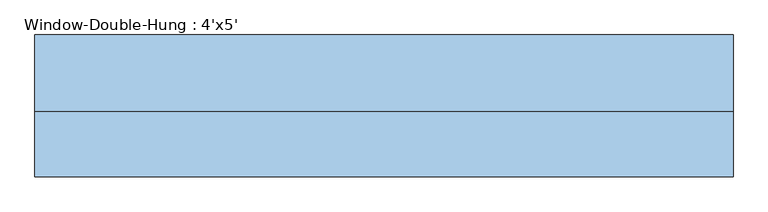
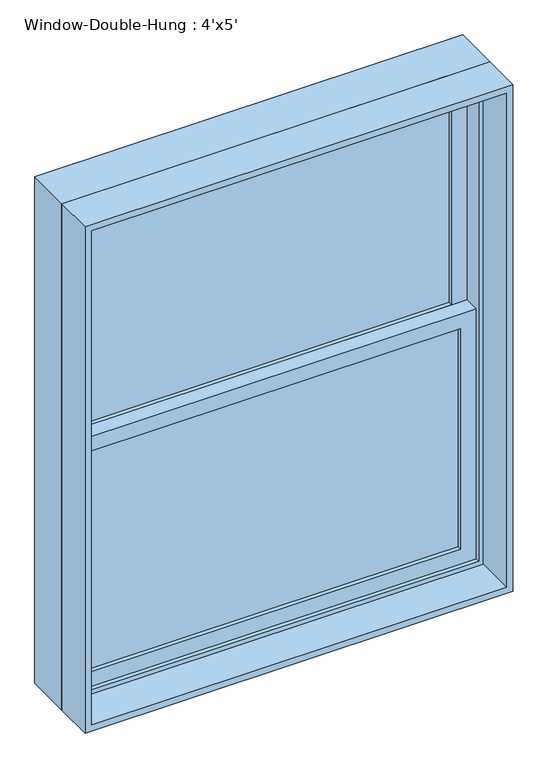
"""IFC4 building model written with IfcOpenShell, lengths in millimetres: window geometry, Window-Double-Hung : 4'x5'."""

from ifc_helpers import new_model, si_unit, frame, origin, place, context, project, spatial, polyline, outline, extrude, source, transform, mapped, element, save


def window_double_hung_4_x5_5ded1df2(model_context):
    return source(origin(), model_context, "Body", "SweptSolid", [
        extrude(outline(polyline([(533.4, 44.45), (533.4, 38.1), (-533.4, 38.1), (-533.4, 44.45), (533.4, 44.45)])), frame((0.0, 0.0, 990.6), z_axis=(0.0, 0.0, 1.0), x_axis=(1.0, 0.0, 0.0)), (0.0, 0.0, 1.0), 663.575),
        extrude(outline(polyline([(-533.4, 31.75), (533.4, 31.75), (533.4, 25.4), (-533.4, 25.4), (-533.4, 31.75)])), frame((0.0, 0.0, 990.6), z_axis=(0.0, 0.0, 1.0), x_axis=(1.0, 0.0, 0.0)), (0.0, 0.0, 1.0), 663.575),
        extrude(outline(polyline([(533.4, 88.9), (533.4, 82.55), (-533.4, 82.55), (-533.4, 88.9), (533.4, 88.9)])), frame((0.0, 0.0, 1698.625), z_axis=(0.0, 0.0, 1.0), x_axis=(1.0, 0.0, 0.0)), (0.0, 0.0, 1.0), 663.575),
        extrude(outline(polyline([(-533.4, 76.2), (533.4, 76.2), (533.4, 69.85), (-533.4, 69.85), (-533.4, 76.2)])), frame((0.0, 0.0, 1698.625), z_axis=(0.0, 0.0, 1.0), x_axis=(1.0, 0.0, 0.0)), (0.0, 0.0, 1.0), 663.575),
        extrude(outline(polyline([(1698.625, -577.85), (946.15, -577.85), (946.15, 577.85), (1698.625, 577.85), (1698.625, -577.85)]), holes=[polyline([(1654.175, 533.4), (990.6, 533.4), (990.6, -533.4), (1654.175, -533.4), (1654.175, 533.4)])]), frame((0.0, 12.7, 0.0), z_axis=(0.0, 1.0, 0.0), x_axis=(0.0, 0.0, 1.0)), (0.0, 0.0, 1.0), 44.45),
        extrude(outline(polyline([(2406.65, -577.85), (1654.175, -577.85), (1654.175, 577.85), (2406.65, 577.85), (2406.65, -577.85)]), holes=[polyline([(2362.2, 533.4), (1698.625, 533.4), (1698.625, -533.4), (2362.2, -533.4), (2362.2, 533.4)])]), frame((0.0, 57.15, 0.0), z_axis=(0.0, 1.0, 0.0), x_axis=(0.0, 0.0, 1.0)), (0.0, 0.0, 1.0), 44.45),
        extrude(outline(polyline([(2438.4, -609.6), (914.4, -609.6), (914.4, 609.6), (2438.4, 609.6), (2438.4, -609.6)]), holes=[polyline([(2406.65, 577.85), (946.15, 577.85), (946.15, -577.85), (2406.65, -577.85), (2406.65, 577.85)])]), frame((0.0, 0.0, 0.0), z_axis=(0.0, 1.0, 0.0), x_axis=(0.0, 0.0, 1.0)), (0.0, 0.0, 1.0), 133.35),
        extrude(outline(polyline([(2438.4, 609.6), (2438.4, -609.6), (914.4, -609.6), (914.4, 609.6), (2438.4, 609.6)]), holes=[polyline([(2419.35, 590.55), (933.45, 590.55), (933.45, -590.55), (2419.35, -590.55), (2419.35, 590.55)])]), frame((0.0, -114.3, 0.0), z_axis=(0.0, 1.0, 0.0), x_axis=(0.0, 0.0, 1.0)), (0.0, 0.0, 1.0), 114.3),
    ])


if __name__ == "__main__":
    model = new_model("IFC4")
    model_context = context("Model", 3, world=origin())
    ifc_project = project(units=[si_unit("LENGTHUNIT", "METRE", prefix="MILLI")], contexts=[model_context])
    site = spatial("IfcSite", under=ifc_project)
    building = spatial("IfcBuilding", under=site)
    placement = place(None, origin())
    window_double_hung_4_x5_shape = window_double_hung_4_x5_5ded1df2(model_context)
    element("IfcWindow", 1, ObjectType="Window-Double-Hung : 4'x5'", at=placement, inside=building, context=model_context, shape_type="MappedRepresentation", body=[
        mapped(window_double_hung_4_x5_shape, transform((0.0, 0.0, 0.0), x_axis=(1.0, 0.0, 0.0), y_axis=(0.0, 1.0, 0.0), z_axis=(0.0, 0.0, 1.0))),
    ])
    save(model, "model.ifc")

# Revit data of these elements
# Type "Window-Double-Hung : 4'x5'"
#   Type Mark = "27"
#   Fire Rating = "0.5h"
#   Construction Type Id = "DG-DR"
#   Assembly Code = "B2020100"
#   Analytic Construction = "Double glazing - domestic"
#   Wall Thickness [instance default] = 0' - 6"
#   Window Inset [instance default] = 0' - 0"
#   Visual Light Transmittance = 0.81
#   Thermal Resistance (R) = 1.8146 (h·ft²·°F)/BTU
#   Solar Heat Gain Coefficient = 0.76
#   Muntin Width = 3' - 6"
#   Muntin Height = 2' - 2 1/8"
#   Interior Wall Closure [instance default] = 0' - 1 1/2"
#   Rough Width = 4' - 0 1/2"
#   Rough Height = 5' - 0 1/2"
#   Frame Extension [instance default] = 0' - 1 1/4"
#   Exterior Wall Closure [instance default] = 0' - 0 1/2"
#   Extension Jamb [instance default] = 0' - 1 1/2"
#   Heat Transfer Coefficient (U) = 0.5511 BTU/(h·ft²·°F)
#   Height = 5' - 0"
#   Width = 4' - 0"
#   Top Muntin Visibility = yes
#   Indicator Visibility [instance default] = yes
#   Extension Jamb Visibility [instance default] = yes
#   Interior Trim Visibility [instance default] = yes
#   Exterior Trim Visibility [instance default] = yes
#   Define Thermal Properties by = 1
#   Bottom Muntin Visibility = yes
#   Muntin Pattern = Muntin Pattern_2x2 : Muntin Pattern_2x2
#   Interior Trim Material = Wood - Stained
#   Interior Trim = Trim-Window-Interior-Flat : Picture Frame
#   Exterior Trim Material = Clad - White
#   Exterior Trim = Trim-Window-Exterior-Flat : with Sill
#   Glass Panel Material = Glass
#   Exterior Frame Material = Clad - White
#   Interior Frame Material = Wood - Stained
#   Wall Closure = (empty or 0)
# Element 1 (IfcWindow, "Window-Double-Hung : 4'x5'")
#   Wall Thickness = 0' - 9"
#   Extension Jamb = 0' - 4 1/2"
#   Materials on its faces: "Wood - Stained", "Glass", "Clad - White"
# Materials
#   "Wood - Stained": class "Wood", colour RGB 224 178 126, transparency 0, Cost = 0
#   "Clad - White": class "Wood", colour RGB 242 242 238, transparency 0, Cost = 0
#   "Glass": class "Glass", colour RGB 154 182 205, transparency 0.85, Description = "Soda Lime Glass", Cost = 0
